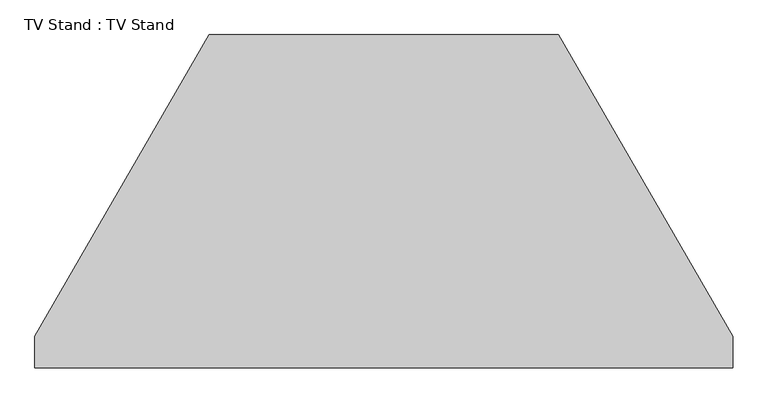
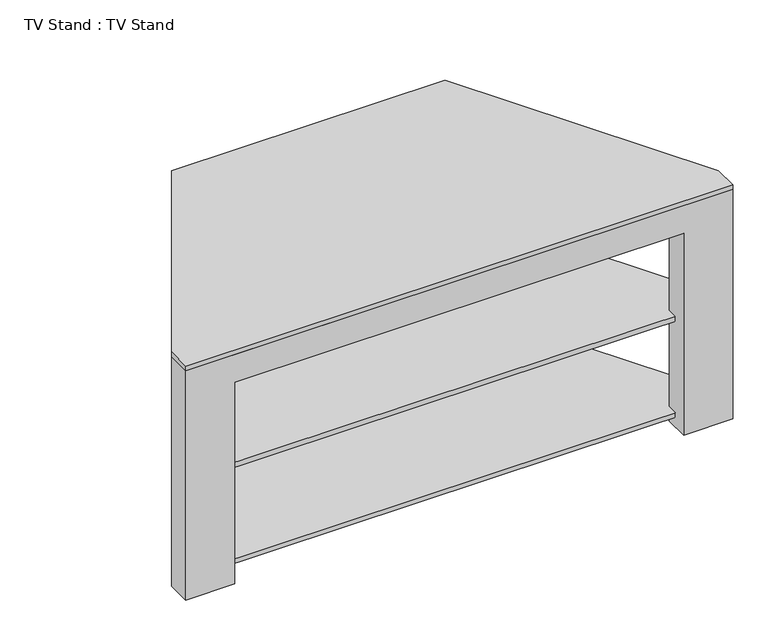
"""IFC4 building model written with IfcOpenShell, lengths in millimetres: furniture geometry, TV Stand : TV Stand."""

from ifc_helpers import new_model, si_unit, point, frame, frame_2d, origin, place, context, project, spatial, polyline, circle_curve, trimmed, segment, composite_curve, outline, extrude, faceted_brep, source, transform, mapped, element, save


def tv_stand_tv_stand_2bc30e45(model_context):
    return source(origin(), model_context, "Body", "SolidModel", [
        extrude(outline(polyline([(421.9276794, -30.0), (633.9880021, -396.8931997), (633.9880021, -503.4), (-383.6119979, -503.4), (-383.6119979, -396.8931997), (-171.5516752, -30.0), (421.9276794, -30.0)])), frame((0.0, 0.0, 20.0), z_axis=(0.0, 0.0, 1.0), x_axis=(1.0, 0.0, 0.0)), (0.0, 0.0, 1.0), 10.0),
        extrude(outline(polyline([(421.9276794, -30.0), (633.9880021, -396.8931997), (633.9880021, -503.4), (-383.6119979, -503.4), (-383.6119979, -396.8931997), (-171.5516752, -30.0), (421.9276794, -30.0)])), frame((0.0, 0.0, 227.65), z_axis=(0.0, 0.0, 1.0), x_axis=(1.0, 0.0, 0.0)), (0.0, 0.0, 1.0), 10.0),
        extrude(outline(polyline([(404.5880021, 0.0), (683.9880021, -483.4), (683.9880021, -533.4), (-433.6119979, -533.4), (-433.6119979, -483.4), (-154.2119979, 0.0), (404.5880021, 0.0)])), frame((0.0, 0.0, 495.3), z_axis=(0.0, 0.0, 1.0), x_axis=(1.0, 0.0, 0.0)), (0.0, 0.0, 1.0), 10.0),
        extrude(outline(polyline([(-50.0, 495.3), (0.0, 495.3), (0.0, 0.0), (-50.0, 0.0), (-50.0, 20.0), (-30.0, 20.0), (-30.0, 30.0), (-50.0, 30.0), (-50.0, 227.65), (-30.0, 227.65), (-30.0, 237.65), (-50.0, 237.65), (-50.0, 495.3)])), frame((-154.2119979, 0.0, 0.0), z_axis=(1.0, 0.0, 0.0), x_axis=(0.0, 1.0, 0.0)), (0.0, 0.0, 1.0), 100.0),
        extrude(outline(polyline([(-50.0, 495.3), (0.0, 495.3), (0.0, 0.0), (-50.0, 0.0), (-50.0, 20.0), (-30.0, 20.0), (-30.0, 30.0), (-50.0, 30.0), (-50.0, 227.65), (-30.0, 227.65), (-30.0, 237.65), (-50.0, 237.65), (-50.0, 495.3)])), frame((304.5880021, 0.0, 0.0), z_axis=(1.0, 0.0, 0.0), x_axis=(0.0, 1.0, 0.0)), (0.0, 0.0, 1.0), 100.0),
        faceted_brep([(-433.6119979, -533.4, 0.0), (-333.6119979, -533.4, 0.0), (-333.6119979, -533.4, 435.3), (583.9880021, -533.4, 435.3), (583.9880021, -533.4, 0.0), (683.9880021, -533.4, 0.0), (683.9880021, -533.4, 495.3), (-433.6119979, -533.4, 495.3), (-433.6119979, -483.4, 0.0), (-433.6119979, -483.4, 495.3), (683.9880021, -483.4, 495.3), (683.9880021, -483.4, 0.0), (583.9880021, -483.4, 0.0), (583.9880021, -483.4, 20.0), (633.9880021, -483.4, 20.0), (633.9880021, -483.4, 30.0), (583.9880021, -483.4, 30.0), (583.9880021, -483.4, 227.65), (633.9880021, -483.4, 227.65), (633.9880021, -483.4, 237.65), (583.9880021, -483.4, 237.65), (583.9880021, -483.4, 435.3), (-333.6119979, -483.4, 435.3), (-333.6119979, -483.4, 237.65), (-383.6119979, -483.4, 237.65), (-383.6119979, -483.4, 227.65), (-333.6119979, -483.4, 227.65), (-333.6119979, -483.4, 30.0), (-383.6119979, -483.4, 30.0), (-383.6119979, -483.4, 20.0), (-333.6119979, -483.4, 20.0), (-333.6119979, -483.4, 0.0), (-333.6119979, -503.4, 20.0), (-333.6119979, -503.4, 30.0), (-333.6119979, -503.4, 227.65), (-333.6119979, -503.4, 237.65), (583.9880021, -503.4, 237.65), (583.9880021, -503.4, 227.65), (583.9880021, -503.4, 30.0), (583.9880021, -503.4, 20.0), (633.9880021, -503.4, 237.65), (-383.6119979, -503.4, 237.65), (-383.6119979, -503.4, 227.65), (633.9880021, -503.4, 227.65), (633.9880021, -503.4, 30.0), (-383.6119979, -503.4, 30.0), (-383.6119979, -503.4, 20.0), (633.9880021, -503.4, 20.0)], [[[0, 1, 2, 3, 4, 5, 6, 7]], [[8, 9, 10, 11, 12, 13, 14, 15, 16, 17, 18, 19, 20, 21, 22, 23, 24, 25, 26, 27, 28, 29, 30, 31]], [[1, 0, 8, 31]], [[2, 1, 31, 30, 32, 33, 27, 26, 34, 35, 23, 22]], [[3, 2, 22, 21]], [[4, 3, 21, 20, 36, 37, 17, 16, 38, 39, 13, 12]], [[5, 4, 12, 11]], [[6, 5, 11, 10]], [[7, 6, 10, 9]], [[0, 7, 9, 8]], [[19, 40, 36, 20]], [[35, 41, 24, 23]], [[25, 42, 34, 26]], [[37, 43, 18, 17]], [[41, 42, 25, 24]], [[42, 41, 35, 34]], [[40, 43, 37, 36]], [[43, 40, 19, 18]], [[15, 44, 38, 16]], [[33, 45, 28, 27]], [[29, 46, 32, 30]], [[39, 47, 14, 13]], [[45, 46, 29, 28]], [[46, 45, 33, 32]], [[44, 47, 39, 38]], [[47, 44, 15, 14]]]),
        extrude(outline(polyline([(0.0, 304.5880021), (495.3, 304.5880021), (495.3, -54.2119979), (0.0, -54.2119979), (0.0, 304.5880021)]), holes=[composite_curve([segment(polyline([(242.65, 145.1700818), (242.65, 105.2059224)]), True, "CONTINUOUS"), segment(trimmed(circle_curve(frame_2d((255.15, 105.2059224)), 12.5), [point((242.65, 105.2059224))], [point((267.65, 105.2059224))], True, "CARTESIAN"), True, "CONTINUOUS"), segment(polyline([(267.65, 105.2059224), (267.65, 145.1700818)]), True, "CONTINUOUS"), segment(trimmed(circle_curve(frame_2d((255.15, 145.1700818)), 12.5), [point((267.65, 145.1700818))], [point((242.65, 145.1700818))], True, "CARTESIAN"), True, "CONTINUOUS")], self_intersect=False), composite_curve([segment(polyline([(35.0, 145.1880021), (35.0, 105.2059224)]), True, "CONTINUOUS"), segment(trimmed(circle_curve(frame_2d((47.5, 105.2059224)), 12.5), [point((35.0, 105.2059224))], [point((60.0, 105.2059224))], True, "CARTESIAN"), True, "CONTINUOUS"), segment(polyline([(60.0, 105.2059224), (60.0, 145.1880021)]), True, "CONTINUOUS"), segment(trimmed(circle_curve(frame_2d((47.5, 145.1880021)), 12.5), [point((60.0, 145.1880021))], [point((35.0, 145.1880021))], True, "CARTESIAN"), True, "CONTINUOUS")], self_intersect=False)]), frame((0.0, -30.0, 0.0), z_axis=(0.0, 1.0, 0.0), x_axis=(0.0, 0.0, 1.0)), (0.0, 0.0, 1.0), 10.0),
    ])


if __name__ == "__main__":
    model = new_model("IFC4")
    model_context = context("Model", 3, world=origin())
    ifc_project = project(units=[si_unit("LENGTHUNIT", "METRE", prefix="MILLI")], contexts=[model_context])
    site = spatial("IfcSite", under=ifc_project)
    building = spatial("IfcBuilding", under=site)
    placement = place(None, origin())
    tv_stand_tv_stand_shape = tv_stand_tv_stand_2bc30e45(model_context)
    element("IfcFurniture", 1, ObjectType="TV Stand : TV Stand", at=placement, inside=building, context=model_context, shape_type="MappedRepresentation", body=[
        mapped(tv_stand_tv_stand_shape, transform((0.0, 0.0, 0.0), x_axis=(1.0, 0.0, 0.0), y_axis=(0.0, 1.0, 0.0), z_axis=(0.0, 0.0, 1.0))),
    ])
    save(model, "model.ifc")

# Revit data of these elements
# Type "TV Stand : TV Stand"
#   Depth = 1' - 9"
#   Width = 3' - 8"
#   Height = 1' - 7 1/2"
#   Finish = Melamine - Gray
#   Default Elevation = 0
# Element 1 (IfcFurniture, "TV Stand : TV Stand")
#   Materials on its faces: "Melamine - Gray", "Glass - Shelves"
# Materials
#   "Melamine - Gray": class "Wood", colour RGB 49 49 49, transparency 0
#   "Glass - Shelves": class "Glass", colour RGB 167 167 167, transparency 0.9
